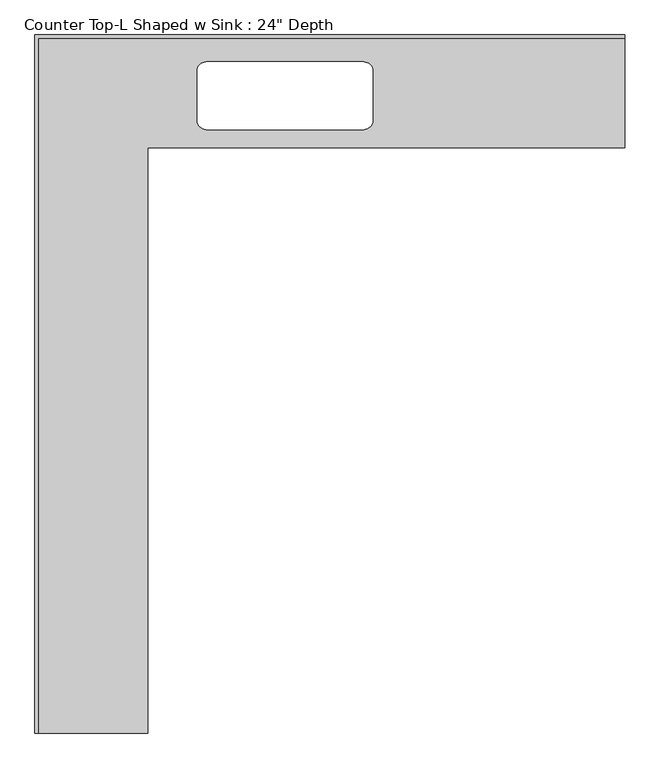
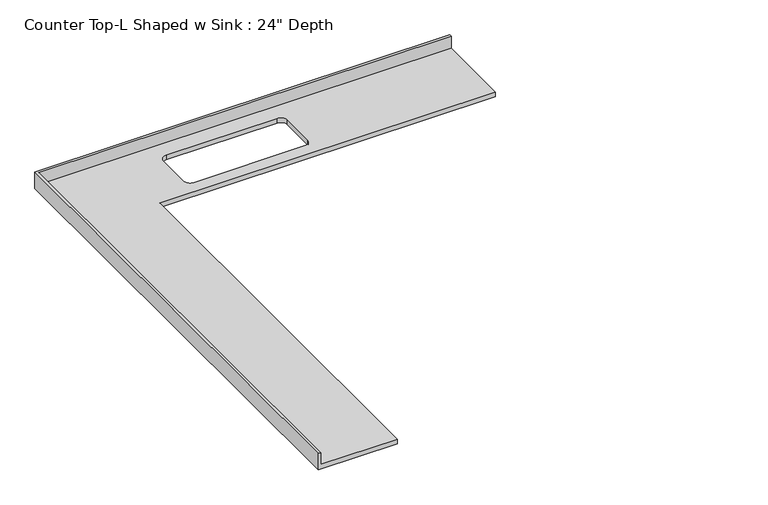
"""IFC4 building model written with IfcOpenShell, lengths in millimetres: furniture geometry."""

from ifc_helpers import new_model, si_unit, frame, origin, place, context, project, spatial, polyline, circle_curve, source, transform, mapped, element, save
from ifc_brep_helpers import plane_surface, revolved_surface, advanced_brep


def furniture_9ea68cb4(model_context):
    return source(origin(), model_context, "Body", "AdvancedBrep", [
        advanced_brep(
        [(-565.4622951, -3937.0, 914.4), (-565.4622951, -635.0, 914.4), (2126.9377049, -635.0, 914.4), (2126.9377049, -19.05, 914.4), (-1181.4122951, -19.05, 914.4), (-1181.4122951, -3937.0, 914.4), (653.7377049, -152.4, 914.4), (704.5377049, -203.2, 914.4), (704.5377049, -482.6, 914.4), (653.7377049, -533.4, 914.4), (-235.2622951, -533.4, 914.4), (-286.0622951, -482.6, 914.4), (-286.0622951, -203.2, 914.4), (-235.2622951, -152.4, 914.4), (2126.9377049, 0.0, 876.3), (2126.9377049, -635.0, 876.3), (-565.4622951, -635.0, 876.3), (-565.4622951, -3937.0, 876.3), (-1200.4622951, -3937.0, 876.3), (-1200.4622951, 0.0, 876.3), (653.7377049, -152.4, 876.3), (-235.2622951, -152.4, 876.3), (-286.0622951, -203.2, 876.3), (-286.0622951, -482.6, 876.3), (-235.2622951, -533.4, 876.3), (653.7377049, -533.4, 876.3), (704.5377049, -482.6, 876.3), (704.5377049, -203.2, 876.3), (-1200.4622951, 0.0, 1016.0), (2126.9377049, 0.0, 1016.0), (-1200.4622951, -3937.0, 1016.0), (-1181.4122951, -3937.0, 1016.0), (2126.9377049, -19.05, 1016.0), (-1181.4122951, -19.05, 1016.0)],
        [
            (0, 1),
            (1, 2),
            (2, 3),
            (3, 4),
            (4, 5),
            (5, 0),
            (6, 7, circle_curve(frame((653.7377049, -203.2, 914.4), z_axis=(0.0, 0.0, -1.0), x_axis=(1.0, 0.0, 0.0)), 50.8)),
            (7, 8),
            (8, 9, circle_curve(frame((653.7377049, -482.6, 914.4), z_axis=(0.0, 0.0, -1.0), x_axis=(1.0, 0.0, 0.0)), 50.8)),
            (9, 10),
            (10, 11, circle_curve(frame((-235.2622951, -482.6, 914.4), z_axis=(0.0, 0.0, -1.0), x_axis=(1.0, 0.0, 0.0)), 50.8)),
            (11, 12),
            (12, 13, circle_curve(frame((-235.2622951, -203.2, 914.4), z_axis=(0.0, 0.0, -1.0), x_axis=(1.0, 0.0, 0.0)), 50.8)),
            (13, 6),
            (14, 15),
            (15, 16),
            (16, 17),
            (17, 18),
            (18, 19),
            (19, 14),
            (20, 21),
            (21, 22, circle_curve(frame((-235.2622951, -203.2, 876.3), z_axis=(0.0, 0.0, 1.0), x_axis=(1.0, 0.0, 0.0)), 50.8)),
            (22, 23),
            (23, 24, circle_curve(frame((-235.2622951, -482.6, 876.3), z_axis=(0.0, 0.0, 1.0), x_axis=(1.0, 0.0, 0.0)), 50.8)),
            (24, 25),
            (25, 26, circle_curve(frame((653.7377049, -482.6, 876.3), z_axis=(0.0, 0.0, 1.0), x_axis=(1.0, 0.0, 0.0)), 50.8)),
            (26, 27),
            (27, 20, circle_curve(frame((653.7377049, -203.2, 876.3), z_axis=(0.0, 0.0, 1.0), x_axis=(1.0, 0.0, 0.0)), 50.8)),
            (19, 28),
            (28, 29),
            (29, 14),
            (18, 30),
            (30, 28),
            (17, 0),
            (5, 31),
            (31, 30),
            (16, 1),
            (15, 2),
            (29, 32),
            (32, 3),
            (6, 20),
            (27, 7),
            (26, 8),
            (25, 9),
            (24, 10),
            (23, 11),
            (22, 12),
            (21, 13),
            (31, 33),
            (33, 32),
            (33, 4),
        ],
        [
            plane_surface(frame((-1200.4622951, 0.0, 914.4), z_axis=(0.0, 0.0, 1.0), x_axis=(-1.0, 0.0, 0.0))),
            plane_surface(frame((-1200.4622951, 0.0, 876.3), z_axis=(0.0, 0.0, -1.0), x_axis=(1.0, 0.0, 0.0))),
            plane_surface(frame((2126.9377049, 0.0, 914.4), z_axis=(0.0, 1.0, 0.0), x_axis=(0.0, 0.0, -1.0))),
            plane_surface(frame((-1200.4622951, 0.0, 914.4), z_axis=(-1.0, 0.0, 0.0), x_axis=(0.0, 0.0, -1.0))),
            plane_surface(frame((-1200.4622951, -3937.0, 914.4), z_axis=(0.0, -1.0, 0.0), x_axis=(0.0, 0.0, -1.0))),
            plane_surface(frame((-565.4622951, -3937.0, 914.4), z_axis=(1.0, 0.0, 0.0), x_axis=(0.0, 0.0, -1.0))),
            plane_surface(frame((-565.4622951, -635.0, 914.4), z_axis=(0.0, -1.0, 0.0), x_axis=(0.0, 0.0, -1.0))),
            plane_surface(frame((2126.9377049, -635.0, 914.4), z_axis=(1.0, 0.0, 0.0), x_axis=(0.0, 0.0, -1.0))),
            revolved_surface(polyline([(704.5377049, -203.2, 876.3), (704.5377049, -203.2, 914.4)]), (653.7377049, -203.2, 0.0), (0.0, 0.0, -1.0)),
            plane_surface(frame((704.5377049, -203.2, 914.4), z_axis=(-1.0, 0.0, 0.0), x_axis=(0.0, 0.0, -1.0))),
            revolved_surface(polyline([(704.5377049, -482.6, 876.3), (704.5377049, -482.6, 914.4)]), (653.7377049, -482.6, 0.0), (0.0, 0.0, -1.0)),
            plane_surface(frame((653.7377049, -533.4, 914.4), z_axis=(0.0, 1.0, 0.0), x_axis=(0.0, 0.0, -1.0))),
            revolved_surface(polyline([(-184.4622951, -482.6, 876.3), (-184.4622951, -482.6, 914.4)]), (-235.2622951, -482.6, 0.0), (0.0, 0.0, -1.0)),
            plane_surface(frame((-286.0622951, -482.6, 914.4), z_axis=(1.0, 0.0, 0.0), x_axis=(0.0, 0.0, -1.0))),
            revolved_surface(polyline([(-184.4622951, -203.2, 876.3), (-184.4622951, -203.2, 914.4)]), (-235.2622951, -203.2, 0.0), (0.0, 0.0, -1.0)),
            plane_surface(frame((-235.2622951, -152.4, 914.4), z_axis=(0.0, -1.0, 0.0), x_axis=(0.0, 0.0, -1.0))),
            plane_surface(frame((-1200.4622951, 0.0, 1016.0), z_axis=(0.0, 0.0, 1.0), x_axis=(0.0, -1.0, 0.0))),
            plane_surface(frame((-1200.4622951, -19.05, 1016.0), z_axis=(0.0, -1.0, 0.0), x_axis=(0.0, 0.0, -1.0))),
            plane_surface(frame((-1181.4122951, -3937.0, 1016.0), z_axis=(1.0, 0.0, 0.0), x_axis=(0.0, 0.0, -1.0))),
        ],
        [
            (0, [[1, 2, 3, 4, 5, 6], [7, 8, 9, 10, 11, 12, 13, 14]]),
            (1, [[15, 16, 17, 18, 19, 20], [21, 22, 23, 24, 25, 26, 27, 28]]),
            (2, [[-20, 29, 30, 31]]),
            (3, [[-19, 32, 33, -29]]),
            (4, [[-32, -18, 34, -6, 35, 36]]),
            (5, [[-1, -34, -17, 37]]),
            (6, [[-2, -37, -16, 38]]),
            (7, [[-15, -31, 39, 40, -3, -38]]),
            (8, [[-7, 41, -28, 42]]),
            (9, [[-8, -42, -27, 43]]),
            (10, [[-9, -43, -26, 44]]),
            (11, [[-10, -44, -25, 45]]),
            (12, [[-11, -45, -24, 46]]),
            (13, [[-12, -46, -23, 47]]),
            (14, [[-13, -47, -22, 48]]),
            (15, [[-14, -48, -21, -41]]),
            (16, [[-33, -36, 49, 50, -39, -30]]),
            (17, [[-40, -50, 51, -4]]),
            (18, [[-49, -35, -5, -51]]),
        ],
    ),
    ])


if __name__ == "__main__":
    model = new_model("IFC4")
    model_context = context("Model", 3, world=origin())
    ifc_project = project(units=[si_unit("LENGTHUNIT", "METRE", prefix="MILLI")], contexts=[model_context])
    site = spatial("IfcSite", under=ifc_project)
    building = spatial("IfcBuilding", under=site)
    placement = place(None, origin())
    furniture_shape = furniture_9ea68cb4(model_context)
    element("IfcFurniture", 1, ObjectType="Counter Top-L Shaped w Sink : 24\" Depth", at=placement, inside=building, context=model_context, shape_type="MappedRepresentation", body=[
        mapped(furniture_shape, transform((0.0, 0.0, 0.0), x_axis=(1.0, 0.0, 0.0), y_axis=(0.0, 1.0, 0.0), z_axis=(0.0, 0.0, 1.0))),
    ])
    save(model, "model.ifc")

# Revit data of these elements
# Type "Counter Top-L Shaped w Sink : 24\" Depth"
#   Assembly Code = "C1030400"
#   Counter Thickness = 0' - 1 1/2"
#   Depth = 2' - 1"
#   Height = 3' - 0"
#   Length - Leg 1 [instance default] = 8' - 0"
#   Length - Leg 2 [instance default] = 6' - 0"
#   Sink Location [instance default] = 3' - 0"
#   Sink Location To Wall [instance default] = 0' - 6"
#   Sink Opening Depth [instance default] = 1' - 3"
#   Sink Opening Width [instance default] = 3' - 3"
#   Counter Top Material = none
#   Default Elevation = 0
# Element 1 (IfcFurniture, "Counter Top-L Shaped w Sink : 24\" Depth")
#   Length - Leg 1 = 10' - 11"
#   Length - Leg 2 = 12' - 11"
#   Materials on its faces: "Counter Top"
# Materials
#   "Counter Top": class "Wood", colour RGB 226 177 128, transparency 0
